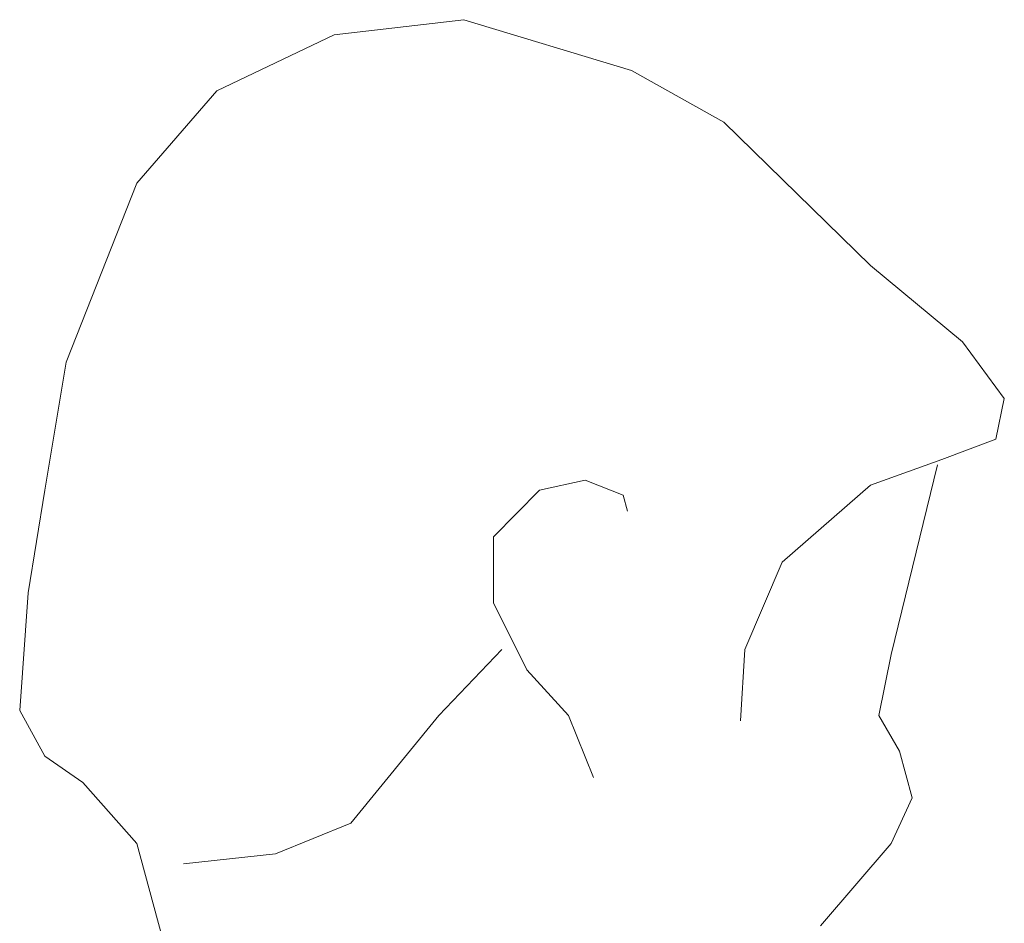
# Model space of a CAD drawing. Units: inches. Extents: x 64 to 1167, y 117 to 939.
# Tile 55 of 56: x 1138.166 to 1146.886, y 495.597 to 503.597. Entities that reach past the tile are written whole.
import ezdxf

# ---------------------------------------------------------------- set-up
doc = ezdxf.new("R2010")
doc.units = ezdxf.units.IN
doc.header["$MEASUREMENT"] = 0
doc.layers.add('A-ENTG', color=8, linetype='Continuous', lineweight=18)

# ---------------------------------------------------------------- blocks, each defined once
blk = doc.blocks.new('A$C43851DCA')
at = {"linetype": 'ByBlock'}
for p, q in [((0.0093942, 0.0669178), (0.008245, 0.0667826)), ((0.0108808, 0.0664672), (0.0093942, 0.0669178)), ((0.008245, 0.0667826), (0.0072064, 0.0662869)), ((0.0116979, 0.0660101), (0.0108808, 0.0664672)), ((0.0072064, 0.0662869), (0.0065, 0.0654693)), ((0.0129948, 0.0647419), (0.0116979, 0.0660101)), ((0.0065, 0.0654693), (0.0058727, 0.0638857)), ((0.0138119, 0.064066), (0.0129948, 0.0647419)), ((0.0141809, 0.0635638), (0.0138119, 0.064066)), ((0.0058727, 0.0638857), (0.0056829, 0.0627527)), ((0.0141071, 0.0632033), (0.0141809, 0.0635638)), ((0.0136274, 0.0630231), (0.0141071, 0.0632033)), ((0.0129948, 0.0627978), (0.0136274, 0.0630231)), ((0.0135905, 0.062978), (0.0131793, 0.0612978)), ((0.0100637, 0.0627527), (0.0104696, 0.0628428)), ((0.0104696, 0.0628428), (0.010807, 0.0627077)), ((0.0122146, 0.0621154), (0.0129948, 0.0627978)), ((0.0056829, 0.0627527), (0.0055353, 0.061845)), ((0.0096578, 0.0623407), (0.0100637, 0.0627527)), ((0.010807, 0.0627077), (0.0108439, 0.062566)), ((0.0096578, 0.0617549), (0.0096578, 0.0623407)), ((0.0118824, 0.0613429), (0.0122146, 0.0621154)), ((0.0055353, 0.061845), (0.0054615, 0.0608022)), ((0.009953, 0.0611627), (0.0096578, 0.0617549)), ((0.0097316, 0.0613429), (0.0091728, 0.0607571)), ((0.0118455, 0.060712), (0.0118824, 0.0613429)), ((0.0131793, 0.0612978), (0.0130686, 0.0607571)), ((0.010322, 0.0607571), (0.009953, 0.0611627)), ((0.0054615, 0.0608022), (0.0056829, 0.0603966)), ((0.0091728, 0.0607571), (0.0083926, 0.0598043)), ((0.0105434, 0.0602099), (0.010322, 0.0607571)), ((0.0130686, 0.0607571), (0.0132531, 0.0604417)), ((0.0132531, 0.0604417), (0.0133638, 0.0600297)), ((0.0056829, 0.0603966), (0.0060203, 0.0601648)), ((0.0060203, 0.0601648), (0.0065, 0.0596241)), ((0.0133638, 0.0600297), (0.0131793, 0.0596241)), ((0.0083926, 0.0598043), (0.0077283, 0.059534)), ((0.0065, 0.0596241), (0.0067214, 0.0588065)), ((0.0131793, 0.0596241), (0.012552, 0.0588967)), ((0.0077283, 0.059534), (0.0069112, 0.0594438))]:
    blk.add_line(p, q, dxfattribs=at)

msp = doc.modelspace()

# ---------------------------------------------------------------- block references
at = {"layer": 'A-ENTG', "xscale": 1000, "yscale": 1000, "zscale": 1000}
msp.add_blockref('A$C43851DCA', (1132.7049, 436.6787), dxfattribs=at)

doc.saveas('drawing.dxf')
